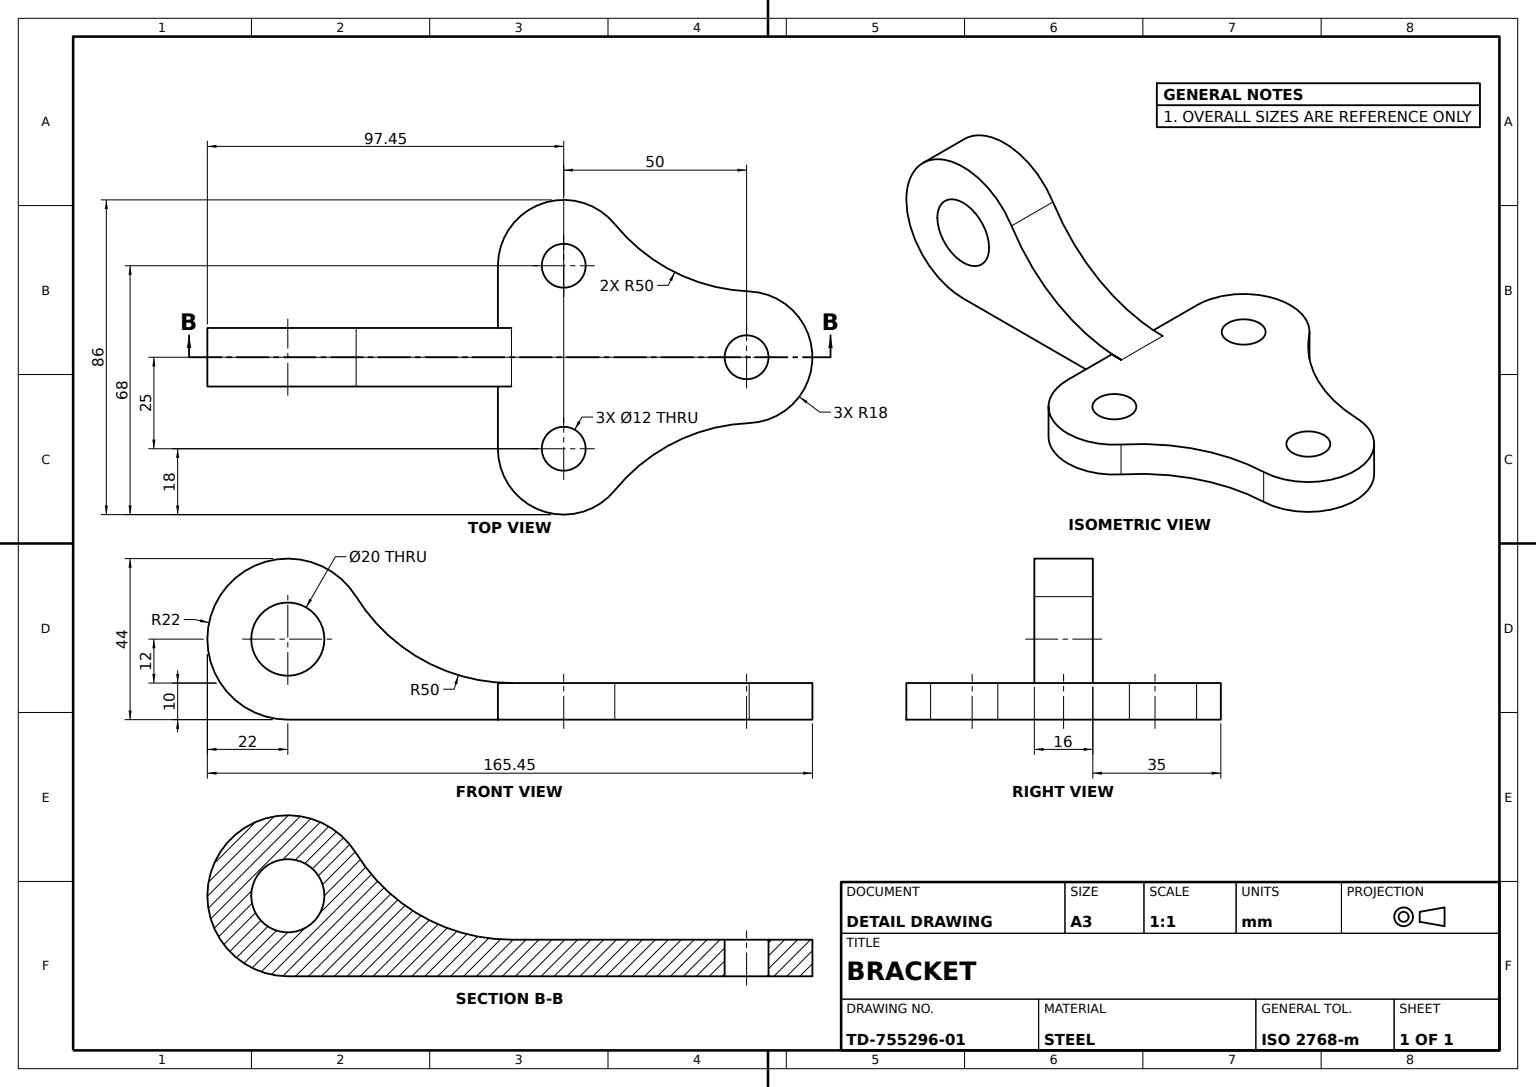
from build123d import *

# Parameters (mm, degrees)
ARM_PROFILE_SKETCH_R     = 10
ARM_BODY_DEPTH           = 8
MOUNTING_FLANGE_SKETCH_R = 6
MOUNTING_FLANGE_DEPTH    = 10
TRIM_CUT_SKETCH_R        = 6
TRIM_CUT_DEPTH           = 117.189881419


with BuildPart() as part:
    # Arm Profile Sketch → Arm Body (new, symmetric)
    with BuildSketch(Plane.XY):
        with BuildLine():
            Line((-41, 0), (86, 0))
            Line((86, 0), (86, 10))
            Line((86, 10), (20.155539406, 10))
            ThreePointArc((20.155539406, 10), (-4.14009349, 16.299631326), (-22.313585182, 33.611111111))
            ThreePointArc((-22.313585182, 33.611111111), (-60.228162216, 32.690078474), (-41, 0))
        make_face()
        with Locations((-41, 22)):
            Circle(ARM_PROFILE_SKETCH_R, mode=Mode.SUBTRACT)
    extrude(amount=ARM_BODY_DEPTH, both=True)

    # Mounting Flange Sketch → Mounting Flange (add)
    with BuildSketch(Plane(origin=(0, 10, 0), x_dir=(1, 0, 0), z_dir=(0, 1, 0))):
        with BuildLine():
            Line((16.445539406, 25), (16.445539406, -25))
            ThreePointArc((16.445539406, -25), (28.412643024, -41.958896227), (48.401557323, -36.367918187))
            ThreePointArc((48.401557323, -36.367918187), (64.807593984, -23.224109156), (85.166263205, -17.985565246))
            ThreePointArc((85.166263205, -17.985565246), (102.445539406, 0), (85.166263205, 17.985565246))
            ThreePointArc((85.166263205, 17.985565246), (64.807593984, 23.224109156), (48.401557323, 36.367918187))
            ThreePointArc((48.401557323, 36.367918187), (28.412643024, 41.958896227), (16.445539406, 25))
        make_face()
        with Locations((84.445539406, 0)):
            Circle(MOUNTING_FLANGE_SKETCH_R, mode=Mode.SUBTRACT)
        with Locations(Location((34.445539406, 25, 0), (0, 0, 270))):
            Circle(MOUNTING_FLANGE_SKETCH_R, mode=Mode.SUBTRACT)
        with Locations(Location((34.445539406, -25, 0), (0, 0, 270))):
            Circle(MOUNTING_FLANGE_SKETCH_R, mode=Mode.SUBTRACT)
    extrude(amount=-MOUNTING_FLANGE_DEPTH)

    # Trim Cut Sketch → Trim Cut (cut, through all)
    with BuildSketch(Plane(origin=(0, 10, 0), x_dir=(1, 0, 0), z_dir=(0, 1, 0))):
        with Locations(Location((84.445539406, 0, 0), (0, 0, 270))):
            Circle(TRIM_CUT_SKETCH_R)
    extrude(amount=-TRIM_CUT_DEPTH, mode=Mode.SUBTRACT)


solid = part.part
